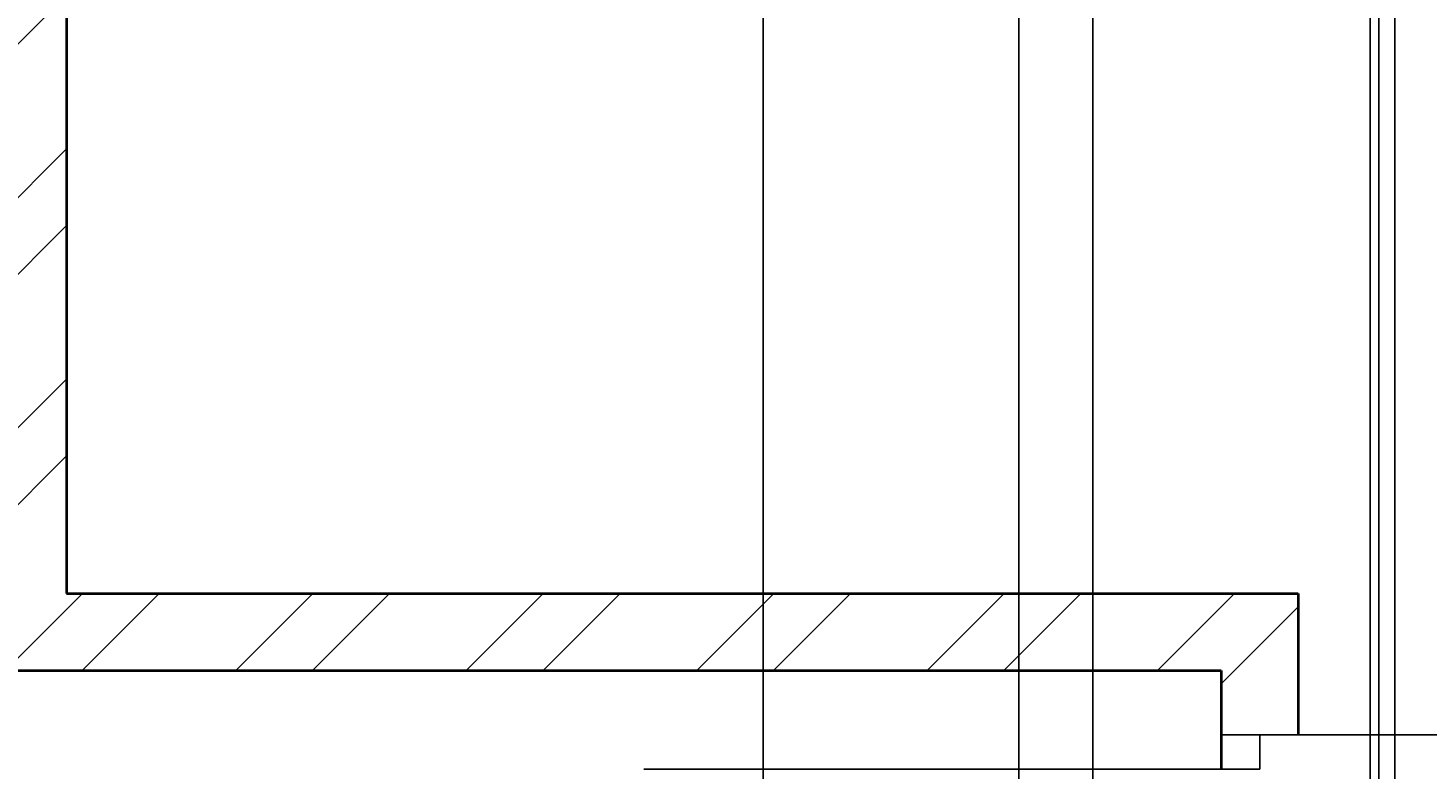
# Model space of a CAD drawing. Units: inches. Extents: x 2063 to 2617, y 1299 to 2210.
# Tile 8 of 22: x 2202 to 2284, y 1858 to 1901. Entities that reach past the tile are written whole.
import ezdxf

# ---------------------------------------------------------------- set-up
doc = ezdxf.new("R2010")
doc.units = ezdxf.units.IN
for name, color, linetype, lineweight in [('A-ANNO-DIMS', 2, 'Continuous', 18), ('A-DOOR', 11, 'Continuous', 25), ('A-WALL', 7, 'Continuous', 40)]:
    doc.layers.add(name, color=color, linetype=linetype, lineweight=lineweight)
doc.layers.add('A-WALL-PATT', color=215, linetype='Continuous', lineweight=13, true_color=0xa953a0)
doc.styles.get("Standard").update_dxf_attribs({"font": 'arial.ttf'})
doc.dimstyles.get("Standard").update_dxf_attribs({"dimtxt": 0.18, "dimasz": 0.18, "dimexe": 0.18, "dimexo": 0.0625, "dimgap": 0.09, "dimtad": 0, "dimtih": 1, "dimtoh": 1, "dimdec": 4, "dimzin": 0, "dimdsep": 46, "dimtxsty": 'Standard', "dimcen": 0.09, "dimadec": 0, "dimazin": 0, "dimtfac": 1, "dimtdec": 4, "dimtofl": 0, "dimtmove": 0, "dimatfit": 3, "dimfxl": 1, "dimtolj": 1, "dimtzin": 0, "dimarcsym": 0})

# ---------------------------------------------------------------- blocks, each defined once
blk = doc.blocks.new('*D50')
at = {"layer": 'A-ANNO-DIMS', "color": 0, "lineweight": -2, "transparency": 16777216}
for p, q in [((2264.144, 2124.25), (2264.144, 1317.702)), ((2280.348, 2124.25), (2280.348, 1317.702)), ((2264.324, 1317.882), (2271.791, 1317.882)), ((2280.168, 1317.882), (2272.701, 1317.882))]:
    blk.add_line(p, q, dxfattribs=at)
at = {"layer": 'A-ANNO-DIMS', "color": 0, "transparency": 16777216}
for points in [[(2264.324, 1317.912), (2264.324, 1317.852), (2264.144, 1317.882)], [(2280.168, 1317.912), (2280.168, 1317.852), (2280.348, 1317.882)]]:
    blk.add_solid(points, dxfattribs=at)
at = {"layer": 'Defpoints', "color": 0, "transparency": 16777216}
for p in [(2264.144, 2124.312), (2280.348, 2124.312), (2280.348, 1317.882)]:
    blk.add_point(p, dxfattribs=at)
at = {"layer": 'A-ANNO-DIMS', "color": 0, "transparency": 16777216, "insert": (2272.246, 1317.882), "char_height": 0.18, "attachment_point": 5}
blk.add_mtext('\\A1;16.204', dxfattribs=at)
blk = doc.blocks.new('*D62')
at = {"layer": 'A-ANNO-DIMS', "color": 0, "lineweight": -2, "transparency": 16777216}
for p, q in [((2259.809, 1437.875), (2259.809, 2170.742)), ((2259.989, 2170.562), (2270.403, 2170.562)), ((2281.608, 2170.562), (2271.194, 2170.562)), ((2281.788, 1437.875), (2281.788, 2170.742))]:
    blk.add_line(p, q, dxfattribs=at)
at = {"layer": 'A-ANNO-DIMS', "color": 0, "transparency": 16777216}
for points in [[(2259.989, 2170.592), (2259.989, 2170.532), (2259.809, 2170.562)], [(2281.608, 2170.592), (2281.608, 2170.532), (2281.788, 2170.562)]]:
    blk.add_solid(points, dxfattribs=at)
at = {"layer": 'Defpoints', "color": 0, "transparency": 16777216}
for p in [(2281.788, 2170.562), (2259.809, 1437.812), (2281.788, 1437.812)]:
    blk.add_point(p, dxfattribs=at)
at = {"layer": 'A-ANNO-DIMS', "color": 0, "transparency": 16777216, "insert": (2270.798, 2170.562), "char_height": 0.18, "attachment_point": 5}
blk.add_mtext('\\A1;21.98', dxfattribs=at)
blk = doc.blocks.new('*D63')
at = {"layer": 'A-ANNO-DIMS', "color": 0, "lineweight": -2, "transparency": 16777216}
for p, q in [((2244.867, 1562.375), (2244.867, 2170.742)), ((2245.047, 2170.562), (2262.4, 2170.562)), ((2280.682, 2170.562), (2263.329, 2170.562)), ((2280.862, 1562.375), (2280.862, 2170.742))]:
    blk.add_line(p, q, dxfattribs=at)
at = {"layer": 'A-ANNO-DIMS', "color": 0, "transparency": 16777216}
for points in [[(2245.047, 2170.592), (2245.047, 2170.532), (2244.867, 2170.562)], [(2280.682, 2170.592), (2280.682, 2170.532), (2280.862, 2170.562)]]:
    blk.add_solid(points, dxfattribs=at)
at = {"layer": 'Defpoints', "color": 0, "transparency": 16777216}
for p in [(2280.862, 2170.562), (2244.867, 1562.312), (2280.862, 1562.312)]:
    blk.add_point(p, dxfattribs=at)
at = {"layer": 'A-ANNO-DIMS', "color": 0, "transparency": 16777216, "insert": (2262.865, 2170.562), "char_height": 0.18, "attachment_point": 5}
blk.add_mtext('\\A1;35.995', dxfattribs=at)
blk = doc.blocks.new('*D69')
at = {"layer": 'A-ANNO-DIMS', "color": 0, "lineweight": -2, "transparency": 16777216}
for p, q in [((2271.707, 1860.051), (2313.574, 1860.051)), ((2313.394, 1859.871), (2313.394, 1845.204)), ((2313.394, 1830.174), (2313.394, 1844.84)), ((2271.707, 1829.994), (2313.574, 1829.994))]:
    blk.add_line(p, q, dxfattribs=at)
at = {"layer": 'A-ANNO-DIMS', "color": 0, "transparency": 16777216}
for points in [[(2313.364, 1859.871), (2313.424, 1859.871), (2313.394, 1860.051)], [(2313.364, 1830.174), (2313.424, 1830.174), (2313.394, 1829.994)]]:
    blk.add_solid(points, dxfattribs=at)
at = {"layer": 'Defpoints', "color": 0, "transparency": 16777216}
for p in [(2271.644, 1860.051), (2271.644, 1829.994), (2313.394, 1829.994)]:
    blk.add_point(p, dxfattribs=at)
at = {"layer": 'A-ANNO-DIMS', "color": 0, "transparency": 16777216, "insert": (2313.394, 1845.022), "char_height": 0.18, "attachment_point": 5}
blk.add_mtext('\\A1;30.057', dxfattribs=at)

msp = doc.modelspace()

# ---------------------------------------------------------------- hatches: boundary and pattern name
at = {"layer": 'A-WALL-PATT'}
h = msp.add_hatch(dxfattribs=at)
h.set_pattern_fill('ANSI32', color=256)
h.paths.add_polyline_path([(2553.6442, 2128.8122), (2511.1703, 2128.8122), (2511.1703, 2124.3122), (2549.1442, 2124.3122), (2549.1442, 2095.662), (2553.6442, 2095.662)])
h.paths.add_polyline_path([(2553.6442, 2035.662), (2549.1442, 2035.662), (2549.1442, 1980.3122), (2503.7214, 1980.3122), (2503.7214, 1975.8122), (2549.1442, 1975.8122), (2549.1442, 1962.9693), (2553.6442, 1962.9693)])
h.paths.add_polyline_path([(2553.6442, 1938.9693), (2549.1442, 1938.9693), (2549.1442, 1927.8122), (2477.1442, 1927.8122), (2477.1442, 1975.8122), (2481.2918, 1975.8122), (2481.2918, 1980.3122), (2453.2648, 1980.3122), (2453.2648, 1975.8122), (2472.6442, 1975.8122), (2472.6442, 1868.3122), (2400.6442, 1868.3122), (2400.6442, 1861.3782), (2405.1442, 1861.3782), (2405.1442, 1863.8122), (2480.9699, 1863.8122), (2480.9699, 1866.0622), (2480.9699, 1868.3122), (2477.1442, 1868.3122), (2477.1442, 1923.3122), (2549.1442, 1923.3122), (2549.1442, 1908.8504), (2553.6442, 1908.8504)])
h.paths.add_polyline_path([(2553.6442, 1884.8504), (2549.1442, 1884.8504), (2549.1442, 1868.3122), (2501.0636, 1868.3122), (2501.0636, 1863.8122), (2549.1442, 1863.8122), (2549.1442, 1826.0298), (2553.6442, 1826.0298)])
h.paths.add_polyline_path([(2388.1504, 1980.3122), (2340.6442, 1980.3122), (2340.6442, 2124.3122), (2358.7501, 2124.3122), (2358.7501, 2128.8122), (2316.3482, 2128.8122), (2316.3482, 2124.3122), (2336.1442, 2124.3122), (2336.1442, 1980.3122), (2289.1737, 1980.3122), (2289.1737, 1975.8122), (2336.1442, 1975.8122), (2336.1442, 1619.3122), (2333.1433, 1619.3122), (2333.1433, 1614.8122), (2344.1671, 1614.8122), (2344.1671, 1617.0622), (2344.1671, 1619.3122), (2340.6442, 1619.3122), (2340.6442, 1975.8122), (2388.1504, 1975.8122), (2388.1504, 1978.0622)])
h.paths.add_polyline_path([(2290.1442, 1614.8122), (2301.4594, 1614.8122), (2301.4594, 1617.0622), (2301.4594, 1619.3122), (2285.6442, 1619.3122), (2285.6442, 1566.8122), (2280.8619, 1566.8122), (2280.8619, 1564.5622), (2280.8619, 1562.3122), (2285.6442, 1562.3122), (2285.6442, 1442.3122), (2281.7879, 1442.3122), (2281.7879, 1437.8122), (2285.6442, 1437.8122), (2285.6442, 1401.8122), (2290.1442, 1401.8122)])
h.paths.add_polyline_path([(2549.1442, 1731.8122), (2405.1442, 1731.8122), (2405.1442, 1834.4638), (2402.8942, 1834.4638), (2400.6442, 1834.4638), (2400.6442, 1727.3122), (2549.1442, 1727.3122)])
h.paths.add_polyline_path([(2553.6442, 1766.0298), (2551.3942, 1766.0298), (2549.1442, 1766.0298), (2549.1442, 1686.7767), (2553.6442, 1686.7767)])
h.paths.add_polyline_path([(2553.6442, 1638.7767), (2551.3942, 1638.7767), (2549.1442, 1638.7767), (2549.1442, 1619.3122), (2448.6442, 1619.3122), (2448.6442, 1610.5671), (2450.8942, 1610.5671), (2453.1442, 1610.5671), (2453.1442, 1614.8122), (2549.1442, 1614.8122), (2549.1442, 1601.6421), (2553.6442, 1601.6421)])
h.paths.add_polyline_path([(2553.6442, 1577.6421), (2551.3942, 1577.6421), (2549.1442, 1577.6421), (2549.1442, 1566.8122), (2453.1442, 1566.8122), (2453.1442, 1591.5045), (2451.0335, 1591.5045), (2448.6442, 1591.5045), (2448.6442, 1566.8122), (2434.0475, 1566.8122), (2434.0475, 1562.3122), (2549.1442, 1562.3122), (2549.1442, 1533.48), (2553.6442, 1533.48)])
h.paths.add_polyline_path([(2553.6442, 1473.48), (2549.1442, 1473.48), (2549.1442, 1442.3122), (2502.6258, 1442.3122), (2502.6258, 1437.8122), (2549.1442, 1437.8122), (2549.1442, 1401.8122), (2553.6442, 1401.8122)])
h.paths.add_polyline_path([(2395.6442, 1562.3122), (2400.0901, 1562.3122), (2400.0901, 1564.5622), (2400.0901, 1566.8122), (2395.6442, 1566.8122), (2395.6442, 1619.3122), (2379.1127, 1619.3122), (2379.1127, 1614.8122), (2391.1442, 1614.8122), (2391.1442, 1401.8122), (2395.6442, 1401.8122), (2395.6442, 1437.8122), (2399.2425, 1437.8122), (2399.2425, 1440.0622), (2399.2425, 1442.3122), (2395.6442, 1442.3122)])
h.paths.add_polyline_path([(2442.6258, 1442.3122), (2419.6262, 1442.3122), (2419.6262, 1437.8122), (2442.6258, 1437.8122), (2442.6258, 1440.0622)])
h.paths.add_polyline_path([(2127.6442, 1480.2532), (2125.3942, 1480.2532), (2123.1442, 1480.2532), (2123.1442, 1401.8122), (2127.6442, 1401.8122), (2127.6442, 1437.8122), (2145.1538, 1437.8122), (2145.1538, 1440.0622), (2145.1538, 1442.3122), (2127.6442, 1442.3122)])
h.paths.add_polyline_path([(2259.809, 1442.3122), (2205.1538, 1442.3122), (2205.1538, 1437.8122), (2259.809, 1437.8122), (2259.809, 1440.0622)])
h.paths.add_polyline_path([(2127.6442, 1659.7652), (2123.1442, 1659.7652), (2123.1442, 1605.5161), (2125.3942, 1605.5161), (2127.6442, 1605.5161), (2127.6442, 1614.8122), (2223.6442, 1614.8122), (2223.6442, 1611.2723), (2228.1442, 1611.2723), (2228.1442, 1619.3122), (2127.6442, 1619.3122)])
h.paths.add_polyline_path([(2244.8673, 1566.8122), (2228.1442, 1566.8122), (2228.1442, 1590.8122), (2225.8942, 1590.8122), (2223.6442, 1590.8122), (2223.6442, 1566.8122), (2127.6442, 1566.8122), (2127.6442, 1581.5161), (2123.1442, 1581.5161), (2123.1442, 1540.2532), (2127.6442, 1540.2532), (2127.6442, 1562.3122), (2244.8673, 1562.3122), (2244.8673, 1564.5622)])
h.paths.add_polyline_path([(2172.5174, 1868.3122), (2127.6442, 1868.3122), (2127.6442, 1886.5833), (2123.1442, 1886.5833), (2123.1442, 1832.6633), (2127.6442, 1832.6633), (2127.6442, 1863.8122), (2172.5174, 1863.8122), (2172.5174, 1866.0622)])
h.paths.add_polyline_path([(2276.1442, 1868.3122), (2204.1442, 1868.3122), (2204.1442, 1923.3122), (2204.1442, 1975.8122), (2224.8362, 1975.8122), (2224.8362, 1978.1097), (2224.8362, 1980.3122), (2195.0729, 1980.3122), (2195.0729, 1978.0622), (2195.0729, 1975.8122), (2199.6442, 1975.8122), (2199.6442, 1927.8122), (2127.6442, 1927.8122), (2127.6442, 1942.3492), (2123.1442, 1942.3492), (2123.1442, 1910.5833), (2127.6442, 1910.5833), (2127.6442, 1923.3122), (2199.6442, 1923.3122), (2199.6442, 1868.3122), (2194.8228, 1868.3122), (2194.8228, 1864.7337), (2194.8228, 1863.8122), (2271.6442, 1863.8122), (2271.6442, 1860.0507), (2276.1442, 1860.0507)])
h.paths.add_polyline_path([(2276.1442, 1829.994), (2273.8942, 1829.994), (2271.6442, 1829.994), (2271.6442, 1731.8122), (2127.6442, 1731.8122), (2127.6442, 1772.6633), (2123.1442, 1772.6633), (2123.1442, 1707.7652), (2127.6442, 1707.7652), (2127.6442, 1727.3122), (2276.1442, 1727.3122)])
h.paths.add_polyline_path([(2127.6442, 2022.1152), (2123.1442, 2022.1152), (2123.1442, 1966.3492), (2127.6442, 1966.3492), (2127.6442, 1975.8122), (2174.2082, 1975.8122), (2174.2082, 1978.0622), (2174.2082, 1980.3122), (2127.6442, 1980.3122)])
h.paths.add_polyline_path([(2361.9755, 1678.588), (2398.4558, 1678.588), (2398.4558, 1697.2453), (2361.9755, 1697.2453)], flags=9)
h.paths.add_polyline_path([(2351.5397, 1780.4072), (2386.1987, 1780.4072), (2386.1987, 1790.7107), (2351.5397, 1790.7107)], flags=25)
h.paths.add_polyline_path([(2350.6753, 1940.9321), (2387.6024, 1940.9321), (2387.6024, 1959.5894), (2350.6753, 1959.5894)], flags=25)
h.paths.add_polyline_path([(2254.9545, 1684.638), (2295.0943, 1684.638), (2295.0943, 1703.2953), (2254.9545, 1703.2953)], flags=9)
h.paths.add_polyline_path([(2282.4946, 1782.4438), (2317.1535, 1782.4438), (2317.1535, 1792.7474), (2282.4946, 1792.7474)], flags=9)
h.paths.add_polyline_path([(2270.327, 1939.2854), (2307.254, 1939.2854), (2307.254, 1957.9428), (2270.327, 1957.9428)], flags=9)

# ---------------------------------------------------------------- linework, layer by layer
at = {"layer": 'A-DOOR'}
for p, q in [((2271.6442, 1860.0507), (2276.1442, 1860.0507)), ((2276.1442, 1860.0507), (2273.8942, 1860.0507)), ((2273.8942, 1860.0507), (2273.8942, 1858.0507)), ((2273.8942, 1858.0507), (2237.8942, 1858.0507))]:
    msp.add_line(p, q, dxfattribs=at)
at = {"layer": 'A-WALL'}
for p, q in [((2204.1442, 1923.3122), (2204.1442, 1868.3122)), ((2204.1442, 1868.3122), (2276.1442, 1868.3122)), ((2276.1442, 1868.3122), (2276.1442, 1860.0507)), ((2194.8228, 1863.8122), (2271.6442, 1863.8122)), ((2271.6442, 1863.8122), (2271.6442, 1858.0507))]:
    msp.add_line(p, q, dxfattribs=at)

# ---------------------------------------------------------------- dimensions: what is measured, and where the dimension line sits
at = {"layer": 'A-ANNO-DIMS'}
for base, p1, p2, override, picture, middle in [((2280.8619, 2170.5622), (2244.8673, 1562.3122), (2280.8619, 1562.3122), {"dimdec": 3, "dimlfac": 1, "dimrnd": 0, "dimzin": 0, "dimdsep": 46, "dimlunit": 2}, '*D63', (2262.8646, 2170.5622)), ((2281.7879, 2170.5622), (2259.809, 1437.8122), (2281.7879, 1437.8122), {"dimdec": 2, "dimlfac": 1, "dimrnd": 0, "dimzin": 0, "dimdsep": 46, "dimlunit": 2}, '*D62', (2270.7984, 2170.5622)), ((2280.3482, 1317.8821), (2264.1442, 2124.3122), (2280.3482, 2124.3122), {"dimdec": 3, "dimlfac": 1, "dimrnd": 0, "dimzin": 0, "dimdsep": 46, "dimlunit": 2}, '*D50', (2272.2462, 1317.8821))]:
    dim = msp.add_linear_dim(base=base, p1=p1, p2=p2, dimstyle='Standard', override=override, dxfattribs=at)
    dim.commit()
    dim.dimension.update_dxf_attribs({"geometry": picture, "text_midpoint": middle})
dim = msp.add_linear_dim(base=(2313.3943, 1829.994), p1=(2271.6442, 1860.0507), p2=(2271.6442, 1829.994), angle=270, dimstyle='Standard', override={"dimdec": 3, "dimlfac": 1, "dimrnd": 0, "dimzin": 0, "dimdsep": 46, "dimlunit": 2}, dxfattribs=at)
dim.commit()
dim.dimension.update_dxf_attribs({"geometry": '*D69', "text_midpoint": (2313.3943, 1845.0224)})

doc.saveas('drawing.dxf')
